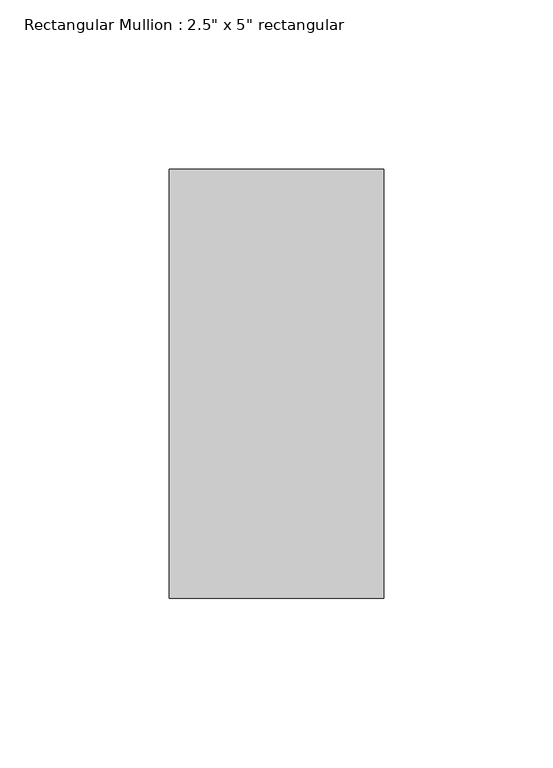
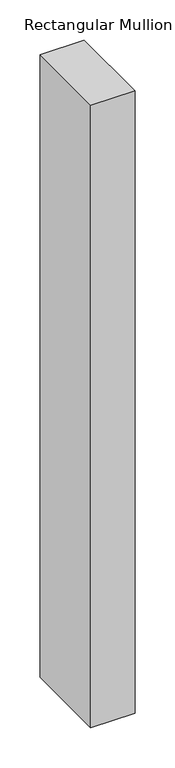
"""IFC4 building model written with IfcOpenShell, lengths in millimetres: member geometry."""

from ifc_helpers import new_model, si_unit, frame, origin, place, context, project, spatial, polyline, outline, extrude, source, transform, mapped, element, save


def member_1988c634(model_context):
    return source(origin(), model_context, "Body", "SweptSolid", [
        extrude(outline(polyline([(31.75, 63.5), (31.75, -63.5), (-31.75, -63.5), (-31.75, 63.5), (31.75, 63.5)])), frame((0.0, 0.0, -948.3113392), z_axis=(0.0, 0.0, 1.0), x_axis=(1.0, 0.0, 0.0)), (0.0, 0.0, 1.0), 948.3113392),
    ])


if __name__ == "__main__":
    model = new_model("IFC4")
    model_context = context("Model", 3, world=origin())
    ifc_project = project(units=[si_unit("LENGTHUNIT", "METRE", prefix="MILLI")], contexts=[model_context])
    site = spatial("IfcSite", under=ifc_project)
    building = spatial("IfcBuilding", under=site)
    placement = place(None, origin())
    member_shape = member_1988c634(model_context)
    element("IfcMember", 1, ObjectType="Rectangular Mullion : 2.5\" x 5\" rectangular", at=placement, inside=building, context=model_context, shape_type="MappedRepresentation", body=[
        mapped(member_shape, transform((0.0, 0.0, 0.0), x_axis=(1.0, 0.0, 0.0), y_axis=(0.0, 1.0, 0.0), z_axis=(0.0, 0.0, 1.0))),
    ])
    save(model, "model.ifc")

# Revit data of these elements
# Type "Rectangular Mullion : 2.5\" x 5\" rectangular"
#   built-in parameter 1007304 = 0.416667 (stored number, unit not read)
#   built-in parameter 1007301 = 0.104167 (stored number, unit not read)
#   built-in parameter 1007300 = 0.104167 (stored number, unit not read)
# Element 1 (IfcMember, "Rectangular Mullion : 2.5\" x 5\" rectangular")
#   Materials on its faces: "Aluminum"
# Materials
#   "Aluminum": class "Metal", colour RGB 247 247 247, transparency 0, Description = "Aluminum 6061", Cost = 0
